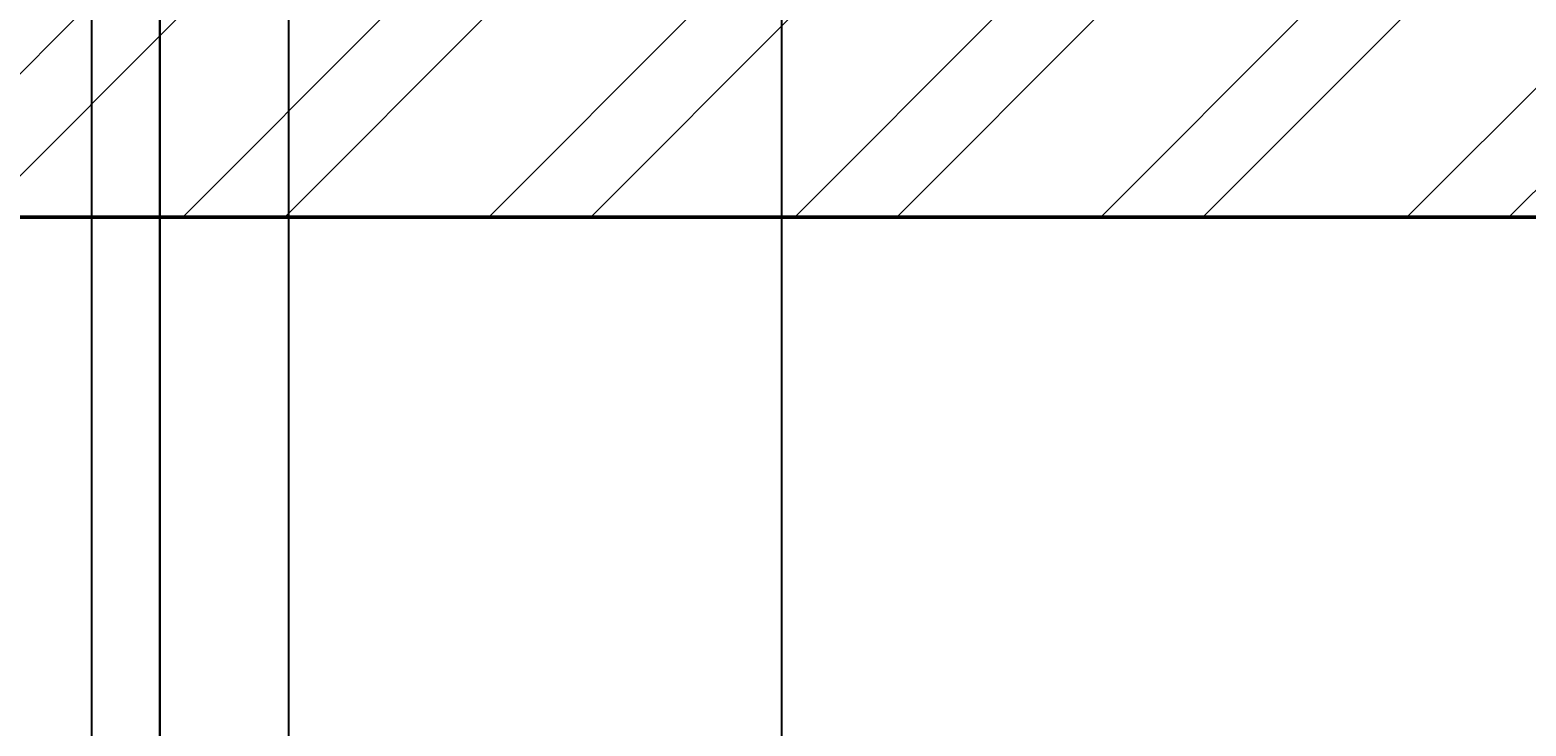
# Model space of a CAD drawing. Units: inches. Extents: x 2812 to 3051, y 1398 to 1659.
# Tile 49 of 65: x 2878 to 2944, y 1528 to 1559. Entities that reach past the tile are written whole.
import ezdxf

# ---------------------------------------------------------------- set-up
doc = ezdxf.new("R2010")
doc.units = ezdxf.units.IN
for name, color, linetype, lineweight in [('A-ANNO-DIMS', 2, 'Continuous', 18), ('S-CONC', 7, 'Continuous', 50), ('S-CONC-PATT', 8, 'Continuous', 18)]:
    doc.layers.add(name, color=color, linetype=linetype, lineweight=lineweight)
doc.styles.get("Standard").update_dxf_attribs({"font": 'arial.ttf'})
doc.dimstyles.get("Standard").update_dxf_attribs({"dimtxt": 0.18, "dimasz": 0.18, "dimexe": 0.18, "dimexo": 0.0625, "dimgap": 0.09, "dimtad": 0, "dimtih": 1, "dimtoh": 1, "dimdec": 4, "dimzin": 0, "dimdsep": 46, "dimtxsty": 'Standard', "dimcen": 0.09, "dimadec": 0, "dimazin": 0, "dimtfac": 1, "dimtdec": 4, "dimtofl": 0, "dimtmove": 0, "dimatfit": 3, "dimfxl": 1, "dimtolj": 1, "dimtzin": 0, "dimarcsym": 0})

# ---------------------------------------------------------------- blocks, each defined once
blk = doc.blocks.new('*D29')
at = {"layer": 'A-ANNO-DIMS', "color": 0, "lineweight": -2, "transparency": 16777216}
for p, q in [((2910.742, 1598.757), (2910.742, 1397.505)), ((2883.385, 1559.757), (2883.385, 1397.505)), ((2883.565, 1397.685), (2896.598, 1397.685)), ((2910.562, 1397.685), (2897.528, 1397.685))]:
    blk.add_line(p, q, dxfattribs=at)
at = {"layer": 'A-ANNO-DIMS', "color": 0, "transparency": 16777216}
for points in [[(2883.565, 1397.715), (2883.565, 1397.655), (2883.385, 1397.685)], [(2910.562, 1397.715), (2910.562, 1397.655), (2910.742, 1397.685)]]:
    blk.add_solid(points, dxfattribs=at)
at = {"layer": 'Defpoints', "color": 0, "transparency": 16777216}
for p in [(2910.742, 1598.82), (2883.385, 1559.82), (2910.742, 1397.685)]:
    blk.add_point(p, dxfattribs=at)
at = {"layer": 'A-ANNO-DIMS', "color": 0, "transparency": 16777216, "insert": (2897.063, 1397.685), "char_height": 0.18, "attachment_point": 5}
blk.add_mtext('\\A1;27.357', dxfattribs=at)
blk = doc.blocks.new('*D58')
at = {"layer": 'A-ANNO-DIMS', "color": 0, "lineweight": -2, "transparency": 16777216}
for p, q in [((2880.385, 1472.098), (2880.385, 1659.35)), ((2880.565, 1659.17), (2881.736, 1659.17)), ((2883.205, 1659.17), (2882.034, 1659.17)), ((2883.385, 1472.098), (2883.385, 1659.35))]:
    blk.add_line(p, q, dxfattribs=at)
at = {"layer": 'A-ANNO-DIMS', "color": 0, "transparency": 16777216}
for points in [[(2880.565, 1659.2), (2880.565, 1659.14), (2880.385, 1659.17)], [(2883.205, 1659.2), (2883.205, 1659.14), (2883.385, 1659.17)]]:
    blk.add_solid(points, dxfattribs=at)
at = {"layer": 'Defpoints', "color": 0, "transparency": 16777216}
for p in [(2883.385, 1659.17), (2880.385, 1472.035), (2883.385, 1472.035)]:
    blk.add_point(p, dxfattribs=at)
at = {"layer": 'A-ANNO-DIMS', "color": 0, "transparency": 16777216, "insert": (2881.885, 1659.17), "char_height": 0.18, "attachment_point": 5}
blk.add_mtext('\\A1;3', dxfattribs=at)
blk = doc.blocks.new('*D59')
at = {"layer": 'A-ANNO-DIMS', "color": 0, "lineweight": -2, "transparency": 16777216}
for p, q in [((2883.385, 1452.098), (2883.385, 1659.35)), ((2883.565, 1659.17), (2885.828, 1659.17)), ((2888.878, 1659.17), (2886.615, 1659.17)), ((2889.058, 1467.465), (2889.058, 1659.35))]:
    blk.add_line(p, q, dxfattribs=at)
at = {"layer": 'A-ANNO-DIMS', "color": 0, "transparency": 16777216}
for points in [[(2883.565, 1659.2), (2883.565, 1659.14), (2883.385, 1659.17)], [(2888.878, 1659.2), (2888.878, 1659.14), (2889.058, 1659.17)]]:
    blk.add_solid(points, dxfattribs=at)
at = {"layer": 'Defpoints', "color": 0, "transparency": 16777216}
for p in [(2889.058, 1659.17), (2889.058, 1467.402), (2883.385, 1452.035)]:
    blk.add_point(p, dxfattribs=at)
at = {"layer": 'A-ANNO-DIMS', "color": 0, "transparency": 16777216, "insert": (2886.221, 1659.17), "char_height": 0.18, "attachment_point": 5}
blk.add_mtext('\\A1;5.673', dxfattribs=at)

msp = doc.modelspace()

# ---------------------------------------------------------------- hatches: boundary and pattern name
at = {"layer": 'S-CONC-PATT'}
h = msp.add_hatch(dxfattribs=at)
h.set_pattern_fill('ANSI32', color=256)
h.paths.add_polyline_path([(3027.3849, 1646.82), (2835.3849, 1646.82), (2835.3849, 1603.2296), (2844.3849, 1603.2296), (2844.3849, 1637.82), (3018.3849, 1637.82), (3018.3849, 1602.5441), (3027.3849, 1602.5441)])
h.paths.add_polyline_path([(2844.3849, 1594.2296), (2835.3849, 1594.2296), (2835.3849, 1550.82), (3027.3849, 1550.82), (3027.3849, 1593.5441), (3018.3849, 1593.5441), (3018.3849, 1559.82), (2844.3849, 1559.82)])
h.paths.add_polyline_path([(2844.3849, 1482.0354), (2835.3849, 1482.0354), (2835.3849, 1463.4959), (2844.3849, 1463.4959)])
h.paths.add_polyline_path([(2844.3849, 1461.4959), (2835.3849, 1461.4959), (2835.3849, 1416.0354), (2844.3849, 1416.0354)])
h.paths.add_polyline_path([(3027.3849, 1482.0354), (3018.3849, 1482.0354), (3018.3849, 1463.2854), (3027.3849, 1463.2854)])
h.paths.add_polyline_path([(3027.3849, 1461.2854), (3018.3849, 1461.2854), (3018.3849, 1416.0354), (3027.3849, 1416.0354)])
h.paths.add_polyline_path([(2961.3849, 1448.4738), (2952.3849, 1448.4738), (2952.3849, 1416.0354), (2961.3849, 1416.0354)])
h.paths.add_polyline_path([(2961.3849, 1462.3026), (2952.3849, 1462.3026), (2952.3849, 1450.4738), (2961.3849, 1450.4738)])
h.paths.add_polyline_path([(2961.3849, 1472.0354), (2952.3849, 1472.0354), (2952.3849, 1462.3026), (2961.3849, 1462.3026)])

# ---------------------------------------------------------------- linework, layer by layer
at = {"layer": 'S-CONC'}
msp.add_line((3027.3849, 1550.82), (2835.3849, 1550.82), dxfattribs=at)

# ---------------------------------------------------------------- dimensions: what is measured, and where the dimension line sits
at = {"layer": 'A-ANNO-DIMS'}
for base, p1, p2, override, picture, middle in [((2883.3849, 1659.17), (2880.3849, 1472.0354), (2883.3849, 1472.0354), {"dimdec": 0, "dimlfac": 1, "dimrnd": 0, "dimzin": 0, "dimdsep": 46, "dimlunit": 2}, '*D58', (2881.8849, 1659.17)), ((2889.0577, 1659.17), (2883.3849, 1452.0354), (2889.0577, 1467.4024), {"dimdec": 3, "dimlfac": 1, "dimrnd": 0, "dimzin": 0, "dimdsep": 46, "dimlunit": 2}, '*D59', (2886.2213, 1659.17)), ((2910.7415, 1397.6854), (2883.3849, 1559.82), (2910.7415, 1598.82), {"dimdec": 3, "dimlfac": 1, "dimrnd": 0, "dimzin": 0, "dimdsep": 46, "dimlunit": 2}, '*D29', (2897.0632, 1397.6854))]:
    dim = msp.add_linear_dim(base=base, p1=p1, p2=p2, dimstyle='Standard', override=override, dxfattribs=at)
    dim.commit()
    dim.dimension.update_dxf_attribs({"geometry": picture, "text_midpoint": middle})

doc.saveas('drawing.dxf')
